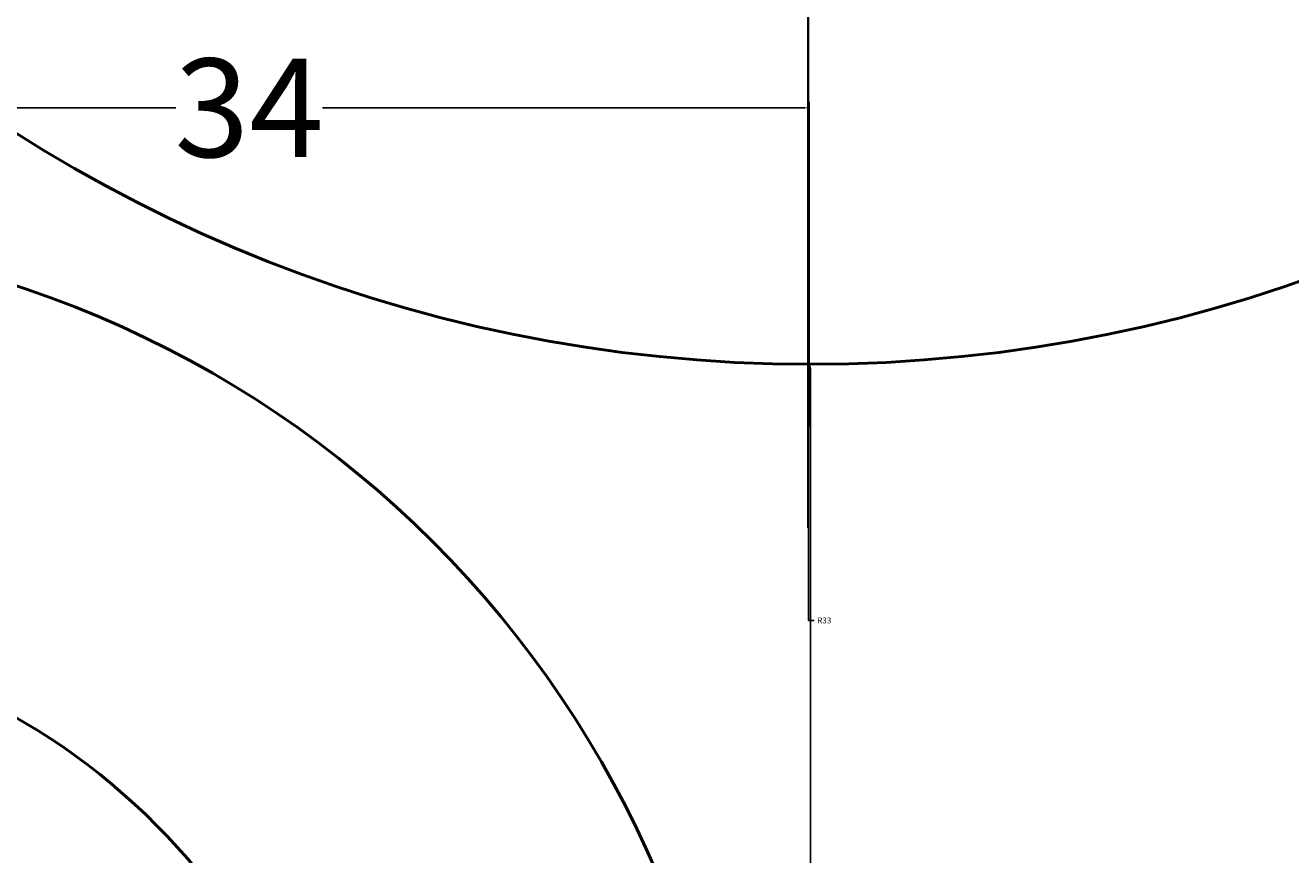
# Model space of a CAD drawing. Units: millimetres. Extents: x -50 to 109, y -46 to 152.
# Tile 8 of 18: x 9 to 48, y 6 to 32. Entities that reach past the tile are written whole.
import ezdxf

# ---------------------------------------------------------------- set-up
doc = ezdxf.new("R2010")
doc.units = ezdxf.units.MM
doc.header["$MEASUREMENT"] = 0
doc.linetypes.add('CENTER', pattern=[50.8, 31.75, -6.35, 6.35, -6.35])
for name, color, linetype, lineweight in [('M-CNTR', 1, 'CENTER', 18), ('M-DIMS', 2, 'Continuous', 25), ('M-OUTL', 7, 'Continuous', 50)]:
    doc.layers.add(name, color=color, linetype=linetype, lineweight=lineweight)
doc.styles.get("Standard").update_dxf_attribs({"font": 'arial.ttf'})
doc.dimstyles.get("Standard").update_dxf_attribs({"dimtxt": 0.18, "dimasz": 0.18, "dimexe": 0.18, "dimexo": 0.0625, "dimgap": 0.09, "dimtad": 0, "dimtih": 1, "dimtoh": 1, "dimdec": 4, "dimzin": 0, "dimdsep": 46, "dimtxsty": 'Standard', "dimcen": 0.09, "dimadec": 0, "dimazin": 0, "dimtfac": 1, "dimtdec": 4, "dimtofl": 0, "dimtmove": 0, "dimatfit": 3, "dimfxl": 1, "dimtolj": 1, "dimtzin": 0, "dimarcsym": 0})

# ---------------------------------------------------------------- blocks, each defined once
blk = doc.blocks.new('*U3')
at = {"layer": 'M-CNTR', "color": 0, "transparency": 16777216}
blk.add_line((0, -85.984), (0, -2.6), dxfattribs=at)
blk = doc.blocks.new('*D18')
at = {"layer": 'Defpoints', "color": 0, "transparency": 16777216}
for p in [(33.131, 66.25), (59.909, 46.965)]:
    blk.add_point(p, dxfattribs=at)
at = {"layer": 'M-DIMS', "color": 0, "lineweight": -2, "transparency": 16777216}
for p, q in [((33.041, 66.25), (33.221, 66.25)), ((33.131, 66.16), (33.131, 66.34)), ((80.717, 31.98), (60.055, 46.86)), ((80.897, 31.98), (80.717, 31.98))]:
    blk.add_line(p, q, dxfattribs=at)
at = {"layer": 'M-DIMS', "color": 0, "transparency": 16777216}
blk.add_solid([(60.073, 46.884), (60.038, 46.835), (59.909, 46.965)], dxfattribs=at)
at = {"layer": 'M-DIMS', "color": 0, "transparency": 16777216, "insert": (84.571, 31.98), "char_height": 0.18, "attachment_point": 5}
blk.add_mtext('\\A1;{\\H16.66667x;R33}', dxfattribs=at)
blk = doc.blocks.new('*D19')
at = {"layer": 'Defpoints', "color": 0, "transparency": 16777216}
for p in [(33.152, 29.059), (-0.925, 20.297), (33.152, 19.299)]:
    blk.add_point(p, dxfattribs=at)
at = {"layer": 'M-DIMS', "color": 0, "lineweight": -2, "transparency": 16777216}
for p, q in [((-0.925, 20.359), (-0.925, 29.239)), ((-0.745, 29.059), (13.882, 29.059)), ((32.972, 29.059), (18.345, 29.059)), ((33.152, 19.361), (33.152, 29.239))]:
    blk.add_line(p, q, dxfattribs=at)
at = {"layer": 'M-DIMS', "color": 0, "transparency": 16777216}
for points in [[(-0.745, 29.089), (-0.745, 29.029), (-0.925, 29.059)], [(32.972, 29.089), (32.972, 29.029), (33.152, 29.059)]]:
    blk.add_solid(points, dxfattribs=at)
at = {"layer": 'M-DIMS', "color": 0, "transparency": 16777216, "insert": (16.113, 29.059), "char_height": 0.18, "attachment_point": 5}
blk.add_mtext('\\A1;{\\H16.66667x;34}', dxfattribs=at)
blk = doc.blocks.new('*D23')
at = {"layer": 'Defpoints', "color": 0, "transparency": 16777216}
for p in [(24.75, 12.317), (-26.598, -25.885)]:
    blk.add_point(p, dxfattribs=at)
at = {"layer": 'M-DIMS', "color": 0, "lineweight": -2, "transparency": 16777216}
for p, q in [((-1.014, -6.784), (-0.834, -6.784)), ((-0.924, -6.874), (-0.924, -6.694)), ((-30.604, -28.865), (-26.742, -25.992)), ((-30.784, -28.865), (-30.604, -28.865))]:
    blk.add_line(p, q, dxfattribs=at)
at = {"layer": 'M-DIMS', "color": 0, "transparency": 16777216}
blk.add_solid([(-26.76, -25.968), (-26.724, -26.016), (-26.598, -25.885)], dxfattribs=at)
at = {"layer": 'M-DIMS', "color": 0, "transparency": 16777216, "insert": (-34.648, -28.865), "char_height": 0.18, "attachment_point": 5}
blk.add_mtext('\\A1;{\\H16.66667x;%%C64}', dxfattribs=at)
blk = doc.blocks.new('*D29')
at = {"layer": 'Defpoints', "color": 0, "transparency": 16777216}
for p in [(21.684, 15.863), (-23.531, -29.431)]:
    blk.add_point(p, dxfattribs=at)
at = {"layer": 'M-DIMS', "color": 0, "lineweight": -2, "transparency": 16777216}
for p, q in [((-1.014, -6.784), (-0.834, -6.784)), ((-0.924, -6.874), (-0.924, -6.694)), ((-37.096, -43.02), (-23.658, -29.559)), ((-37.276, -43.02), (-37.096, -43.02))]:
    blk.add_line(p, q, dxfattribs=at)
at = {"layer": 'M-DIMS', "color": 0, "transparency": 16777216}
blk.add_solid([(-23.68, -29.537), (-23.637, -29.58), (-23.531, -29.431)], dxfattribs=at)
at = {"layer": 'M-DIMS', "color": 0, "transparency": 16777216, "insert": (-37.592, -43.02), "char_height": 0.18, "attachment_point": 5}
blk.add_mtext('\\A1;∅64', dxfattribs=at)
blk = doc.blocks.new('*D38')
at = {"layer": 'Defpoints', "color": 0, "transparency": 16777216}
for p in [(33.131, 66.25), (33.131, 33.25)]:
    blk.add_point(p, dxfattribs=at)
at = {"layer": 'M-DIMS', "color": 0, "lineweight": -2, "transparency": 16777216}
for p, q in [((33.041, 66.25), (33.221, 66.25)), ((33.131, 66.16), (33.131, 66.34)), ((33.131, 13.45), (33.131, 33.07)), ((33.311, 13.45), (33.131, 13.45))]:
    blk.add_line(p, q, dxfattribs=at)
at = {"layer": 'M-DIMS', "color": 0, "transparency": 16777216}
blk.add_solid([(33.161, 33.07), (33.101, 33.07), (33.131, 33.25)], dxfattribs=at)
at = {"layer": 'M-DIMS', "color": 0, "transparency": 16777216, "insert": (33.616, 13.45), "char_height": 0.18, "attachment_point": 5}
blk.add_mtext('\\A1;R33', dxfattribs=at)
blk = doc.blocks.new('*D39')
at = {"layer": 'Defpoints', "color": 0, "transparency": 16777216}
for p in [(33.197, 66.25), (33.197, 21.25)]:
    blk.add_point(p, dxfattribs=at)
at = {"layer": 'M-DIMS', "color": 0, "lineweight": -2, "transparency": 16777216}
for p, q in [((33.107, 66.25), (33.287, 66.25)), ((33.197, 66.16), (33.197, 66.34)), ((33.197, -5.75), (33.197, 21.07)), ((33.017, -5.75), (33.197, -5.75))]:
    blk.add_line(p, q, dxfattribs=at)
at = {"layer": 'M-DIMS', "color": 0, "transparency": 16777216}
blk.add_solid([(33.167, 21.07), (33.227, 21.07), (33.197, 21.25)], dxfattribs=at)
at = {"layer": 'M-DIMS', "color": 0, "transparency": 16777216, "insert": (32.711, -5.75), "char_height": 0.18, "attachment_point": 5}
blk.add_mtext('\\A1;R45', dxfattribs=at)

msp = doc.modelspace()

# ---------------------------------------------------------------- linework, layer by layer
at = {"layer": 'M-OUTL'}
msp.add_circle((-0.92366, -6.78396), 32, dxfattribs=at)
for centre, radius, start, end in [((33.197, 66.24997), 45, 180.010473, 359.989527), ((-0.91099, -6.86447), 20, 32.692944, 75.356698)]:
    msp.add_arc(centre, radius, start, end, dxfattribs=at)

# ---------------------------------------------------------------- block references
at = {"layer": 'M-CNTR'}
msp.add_blockref('*U3', (33.11888, 102.25066), dxfattribs=at)

# ---------------------------------------------------------------- dimensions: what is measured, and where the dimension line sits
at = {"layer": 'M-DIMS'}
for center, mpoint, picture, middle in [((33.197, 66.24997), (33.197, 21.24997), '*D39', (32.71127, -5.75003)), ((33.1307, 66.24997), (33.131, 33.24997), '*D38', (33.61623, 13.44997))]:
    dim = msp.add_radius_dim(center=center, mpoint=mpoint, dimstyle='Standard', override={"dimdec": 0, "dimlfac": 1, "dimrnd": 0, "dimzin": 0, "dimdsep": 46, "dimlunit": 2}, dxfattribs=at)
    dim.commit()
    dim.dimension.update_dxf_attribs({"geometry": picture, "text_midpoint": middle, "dimtype": 164})
dim = msp.add_radius_dim(center=(33.1307, 66.24997), mpoint=(59.90911, 46.96483), text='{\\H16.66667x;R33}', dimstyle='Standard', override={"dimclrd": 0, "dimclre": 0, "dimclrt": 0}, dxfattribs=at)
dim.commit()
dim.dimension.update_dxf_attribs({"geometry": '*D18', "text_midpoint": (84.57118, 31.97955), "dimtype": 164})
dim = msp.add_linear_dim(base=(33.15184, 29.05873), p1=(-0.92498, 20.29688), p2=(33.15184, 19.29869), text='{\\H16.66667x;34}', dimstyle='Standard', override={"dimclrd": 0, "dimclre": 0, "dimclrt": 0}, dxfattribs=at)
dim.commit()
dim.dimension.update_dxf_attribs({"geometry": '*D19', "text_midpoint": (16.11343, 29.05873)})
dim = msp.add_diameter_dim_2p(p1=(21.68387, 15.86332), p2=(-23.53119, -29.43125), dimstyle='Standard', override={"dimdec": 0, "dimlfac": 1, "dimrnd": 0, "dimzin": 0, "dimdsep": 46, "dimlunit": 2}, dxfattribs=at)
dim.commit()
dim.dimension.update_dxf_attribs({"geometry": '*D29', "text_midpoint": (-37.59218, -43.01962), "dimtype": 163})
dim = msp.add_diameter_dim_2p(p1=(24.75033, 12.31698), p2=(-26.59765, -25.88491), text='{\\H16.66667x;%%C64}', dimstyle='Standard', override={"dimclrd": 0, "dimclre": 0, "dimclrt": 0}, dxfattribs=at)
dim.commit()
dim.dimension.update_dxf_attribs({"geometry": '*D23', "text_midpoint": (-34.64806, -28.86518), "dimtype": 163})

doc.saveas('drawing.dxf')
